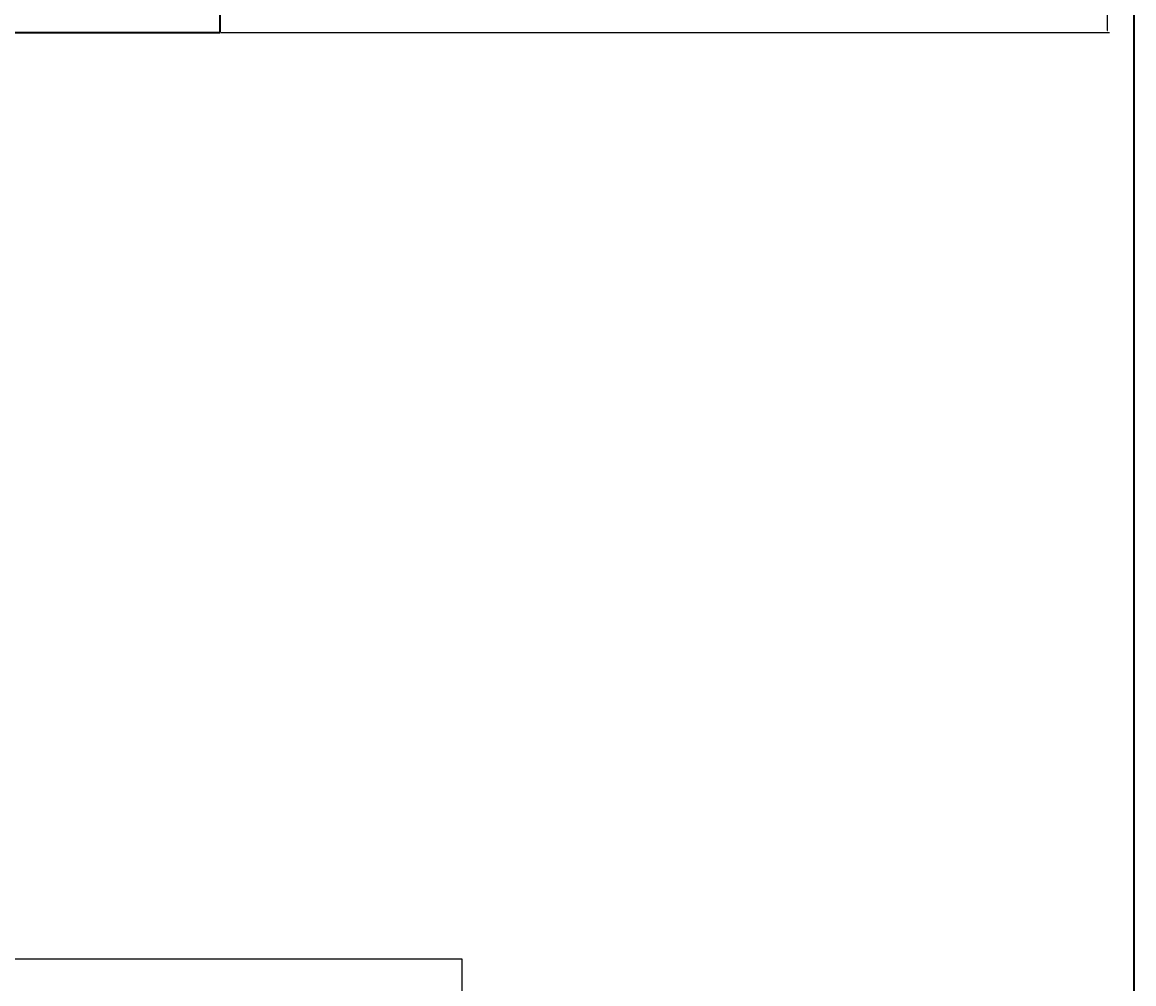
# Model space of a CAD drawing. Units: inches. Extents: x 1088 to 1703, y 668 to 1875.
# Tile 7 of 45: x 1602 to 1703, y 1329 to 1416. Entities that reach past the tile are written whole.
import ezdxf

# ---------------------------------------------------------------- set-up
doc = ezdxf.new("R2010")
doc.units = ezdxf.units.IN
for name, color, linetype, lineweight in [('A-ANNO-DIMS', 2, 'Continuous', 18), ('A-ANNO-TTLB', 7, 'Continuous', 35), ('A-FLOR-HRAL', 7, 'Continuous', 25), ('A-WALL', 7, 'Continuous', 35)]:
    doc.layers.add(name, color=color, linetype=linetype, lineweight=lineweight)
doc.styles.get("Standard").update_dxf_attribs({"font": 'arial.ttf'})
doc.dimstyles.get("Standard").update_dxf_attribs({"dimtxt": 0.18, "dimasz": 0.18, "dimexe": 0.18, "dimexo": 0.0625, "dimgap": 0.09, "dimtad": 0, "dimtih": 1, "dimtoh": 1, "dimdec": 4, "dimzin": 0, "dimdsep": 46, "dimtxsty": 'Standard', "dimcen": 0.09, "dimadec": 0, "dimazin": 0, "dimtfac": 1, "dimtdec": 4, "dimtofl": 0, "dimtmove": 0, "dimatfit": 3, "dimfxl": 1, "dimtolj": 1, "dimtzin": 0, "dimarcsym": 0})

# ---------------------------------------------------------------- blocks, each defined once
blk = doc.blocks.new('*D30')
at = {"layer": 'A-ANNO-DIMS', "color": 0, "lineweight": -2, "transparency": 16777216}
for p, q in [((1624.91, 1803.56), (1700.97, 1803.56)), ((1700.79, 1803.38), (1700.79, 1609.49)), ((1700.79, 1415.24), (1700.79, 1609.13)), ((1620.41, 1415.06), (1700.97, 1415.06))]:
    blk.add_line(p, q, dxfattribs=at)
at = {"layer": 'A-ANNO-DIMS', "color": 0, "transparency": 16777216}
for points in [[(1700.76, 1803.38), (1700.82, 1803.38), (1700.79, 1803.56)], [(1700.76, 1415.24), (1700.82, 1415.24), (1700.79, 1415.06)]]:
    blk.add_solid(points, dxfattribs=at)
at = {"layer": 'Defpoints', "color": 0, "transparency": 16777216}
for p in [(1624.84, 1803.56), (1700.79, 1803.56), (1620.34, 1415.06)]:
    blk.add_point(p, dxfattribs=at)
at = {"layer": 'A-ANNO-DIMS', "color": 0, "transparency": 16777216, "insert": (1700.79, 1609.31), "char_height": 0.18, "attachment_point": 5}
blk.add_mtext('\\A1;388.5', dxfattribs=at)

msp = doc.modelspace()

# ---------------------------------------------------------------- linework, layer by layer
at = {"layer": 'A-ANNO-TTLB'}
msp.add_lwpolyline([(1088.369, 1874.677), (1703.181, 1874.677), (1703.181, 667.947), (1088.369, 667.947)], close=True, dxfattribs=at)
at = {"layer": 'A-FLOR-HRAL'}
for p, q in [((1590.345, 1331.058), (1642.243, 1331.058)), ((1642.243, 1331.058), (1642.243, 1181.058))]:
    msp.add_line(p, q, dxfattribs=at)
at = {"layer": 'A-WALL'}
for p, q in [((1620.345, 1415.058), (1620.345, 1474.363)), ((1590.345, 1415.058), (1614.345, 1415.058)), ((1614.345, 1415.058), (1620.345, 1415.058))]:
    msp.add_line(p, q, dxfattribs=at)

# ---------------------------------------------------------------- dimensions: what is measured, and where the dimension line sits
at = {"layer": 'A-ANNO-DIMS'}
dim = msp.add_linear_dim(base=(1700.793, 1803.558), p1=(1620.345, 1415.058), p2=(1624.845, 1803.558), angle=90, dimstyle='Standard', override={"dimdec": 1, "dimlfac": 1, "dimrnd": 0, "dimzin": 0, "dimdsep": 46, "dimlunit": 2}, dxfattribs=at)
dim.commit()
dim.dimension.update_dxf_attribs({"geometry": '*D30', "text_midpoint": (1700.793, 1609.308)})

doc.saveas('drawing.dxf')
